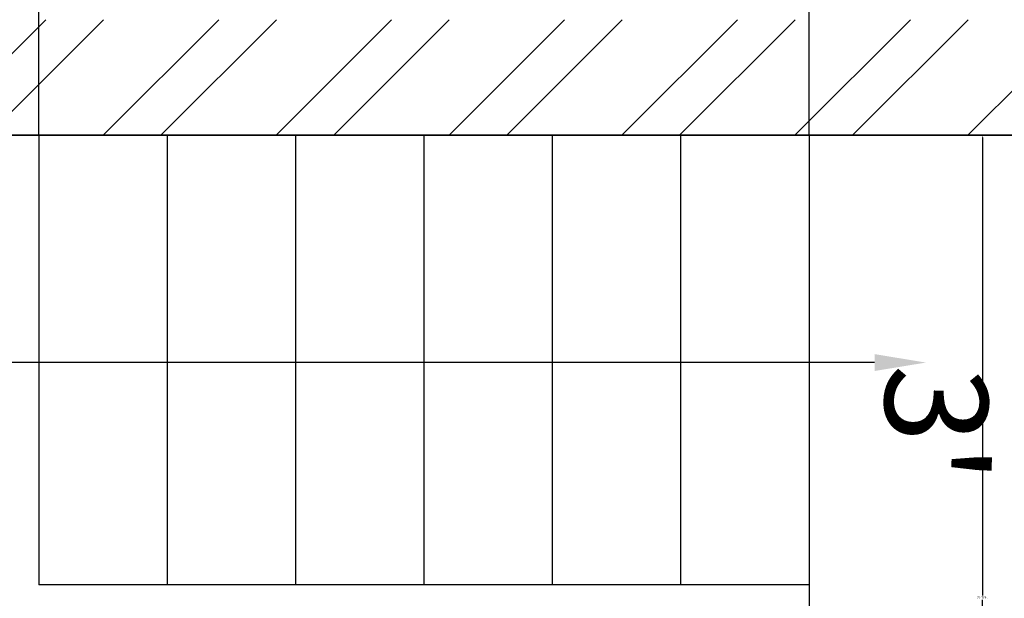
# Model space of a CAD drawing. Units: inches. Extents: x 2166 to 3588, y 1959 to 2628.
# Tile 10 of 13: x 3457 to 3534, y 2067 to 2112. Entities that reach past the tile are written whole.
import ezdxf
from ezdxf import colors
from ezdxf.entities.mleader import LeaderData, LeaderLine
from ezdxf.math import Vec2, Vec3

# ---------------------------------------------------------------- set-up
doc = ezdxf.new("R2010")
doc.units = ezdxf.units.IN
for name, color, linetype, lineweight in [('A-ANNO-DIMS', 2, 'Continuous', 18), ('A-ANNO-SYMB', 136, 'Continuous', 18), ('A-AREA-IDEN', 170, 'Continuous', 18), ('A-WALL-PATT', 20, 'Continuous', 13), ('Staircase', 136, 'Continuous', 25), ('WALL', 40, 'Continuous', 35)]:
    doc.layers.add(name, color=color, linetype=linetype, lineweight=lineweight)
doc.styles.get("Standard").update_dxf_attribs({"font": 'arial.ttf'})
doc.dimstyles.get("Standard").update_dxf_attribs({"dimtxt": 0.18, "dimasz": 0.18, "dimexe": 0.18, "dimexo": 0.0625, "dimgap": 0.09, "dimtad": 0, "dimtih": 1, "dimtoh": 1, "dimdec": 4, "dimzin": 0, "dimdsep": 46, "dimtxsty": 'Standard', "dimcen": 0.09, "dimadec": 0, "dimazin": 0, "dimtfac": 1, "dimtdec": 4, "dimtofl": 0, "dimtmove": 0, "dimatfit": 3, "dimfxl": 1, "dimtolj": 1, "dimtzin": 0, "dimarcsym": 0})

# ---------------------------------------------------------------- blocks, each defined once
blk = doc.blocks.new('STAIR-RETURN-FLIGHTS')
for p, q in [((30, 72), (30, 37)), ((40, 72), (40, 37)), ((50, 72), (50, 37)), ((60, 72), (60, 37)), ((70, 72), (70, 37)), ((80, 72), (80, 37)), ((90, 72), (90, 0)), ((90, 37), (30, 37))]:
    blk.add_line(p, q)
blk = doc.blocks.new('*D18')
at = {"layer": 'A-ANNO-DIMS', "color": 0, "lineweight": -2, "transparency": 16777216}
for p, q in [((3518.533, 2102.979), (3532.151, 2102.979)), ((3531.971, 2102.799), (3531.971, 2067.159)), ((3531.971, 2031.159), (3531.971, 2066.799)), ((3518.533, 2030.979), (3532.151, 2030.979))]:
    blk.add_line(p, q, dxfattribs=at)
at = {"layer": 'A-ANNO-DIMS', "color": 0, "transparency": 16777216}
for points in [[(3531.941, 2102.799), (3532.001, 2102.799), (3531.971, 2102.979)], [(3531.941, 2031.159), (3532.001, 2031.159), (3531.971, 2030.979)]]:
    blk.add_solid(points, dxfattribs=at)
at = {"layer": 'Defpoints', "color": 0, "transparency": 16777216}
for p in [(3518.471, 2102.979), (3531.971, 2102.979), (3518.471, 2030.979)]:
    blk.add_point(p, dxfattribs=at)
at = {"layer": 'A-ANNO-DIMS', "color": 0, "transparency": 16777216, "insert": (3531.971, 2066.979), "char_height": 0.18, "attachment_point": 5}
blk.add_mtext('\\A1;72 TYP.', dxfattribs=at)
blk = doc.blocks.new('*D52')
at = {"layer": 'A-ANNO-DIMS', "color": 0, "lineweight": -2, "transparency": 16777216}
for p, q in [((3458.471, 2103.041), (3458.471, 2127.909)), ((3458.651, 2127.729), (3488.251, 2127.729)), ((3518.291, 2127.729), (3488.69, 2127.729)), ((3518.471, 2103.041), (3518.471, 2127.909))]:
    blk.add_line(p, q, dxfattribs=at)
at = {"layer": 'A-ANNO-DIMS', "color": 0, "transparency": 16777216}
for points in [[(3458.651, 2127.759), (3458.651, 2127.699), (3458.471, 2127.729)], [(3518.291, 2127.759), (3518.291, 2127.699), (3518.471, 2127.729)]]:
    blk.add_solid(points, dxfattribs=at)
at = {"layer": 'Defpoints', "color": 0, "transparency": 16777216}
for p in [(3518.471, 2127.729), (3458.471, 2102.979), (3518.471, 2102.979)]:
    blk.add_point(p, dxfattribs=at)
at = {"layer": 'A-ANNO-DIMS', "color": 0, "transparency": 16777216, "insert": (3488.471, 2127.729), "char_height": 0.18, "attachment_point": 5}
blk.add_mtext('\\A1;60', dxfattribs=at)

msp = doc.modelspace()

# ---------------------------------------------------------------- hatches: boundary and pattern name
at = {"layer": 'A-WALL-PATT'}
h = msp.add_hatch(dxfattribs=at)
h.set_pattern_fill('ANSI32', color=256)
h.paths.add_polyline_path([(3563.471, 2429.979), (3227.471, 2429.979), (3227.471, 2021.979), (3563.471, 2021.979)])
h.paths.add_polyline_path([(3236.471, 2420.979), (3554.471, 2420.979), (3554.471, 2111.979), (3236.471, 2111.979)], flags=16)
h.paths.add_polyline_path([(3236.471, 2102.979), (3554.471, 2102.979), (3554.471, 2030.979), (3236.471, 2030.979)], flags=16)
h.paths.add_polyline_path([(3518.471, 2085.283), (3518.471, 2067.979), (3458.471, 2067.979), (3458.471, 2085.283)], flags=0)
h.paths.add_polyline_path([(3434.656, 2082.283), (3442.194, 2082.283), (3442.194, 2087.514), (3434.656, 2087.514)], flags=8)
h.paths.add_polyline_path([(3522.671, 2094.512), (3521.752, 2052.984), (3545.541, 2052.457), (3546.46, 2093.986)], flags=8)

# ---------------------------------------------------------------- linework, layer by layer
at = {"layer": 'WALL'}
msp.add_line((3554.471, 2102.979), (3236.471, 2102.979), dxfattribs=at)

# ---------------------------------------------------------------- block references
at = {"layer": 'Staircase'}
msp.add_blockref('STAIR-RETURN-FLIGHTS', (3428.471, 2030.979), dxfattribs=at)

# ---------------------------------------------------------------- texts
at = {"layer": 'A-AREA-IDEN', "insert": (3545.955, 2091.996), "char_height": 8, "attachment_point": 1, "rotation": 268.73191}
msp.add_mtext_dynamic_manual_height_columns("{\\Fsuperos|c0;LANDING\\P   3'}", width=58.85395, gutter_width=12.5, heights=[0], dxfattribs=at)

# ---------------------------------------------------------------- dimensions: what is measured, and where the dimension line sits
at = {"layer": 'A-ANNO-DIMS'}
dim = msp.add_linear_dim(base=(3518.471, 2127.729), p1=(3458.471, 2102.979), p2=(3518.471, 2102.979), dimstyle='Standard', override={"dimdec": 0, "dimlfac": 1, "dimrnd": 0, "dimzin": 0, "dimdsep": 46, "dimlunit": 2}, dxfattribs=at)
dim.commit()
dim.dimension.update_dxf_attribs({"geometry": '*D52', "text_midpoint": (3488.471, 2127.729)})
dim = msp.add_linear_dim(base=(3531.971, 2102.979), p1=(3518.471, 2030.979), p2=(3518.471, 2102.979), angle=90, text='<> TYP.', dimstyle='Standard', override={"dimdec": 0, "dimlfac": 1, "dimrnd": 0, "dimzin": 0, "dimdsep": 46, "dimlunit": 2}, dxfattribs=at)
dim.commit()
dim.dimension.update_dxf_attribs({"geometry": '*D18', "text_midpoint": (3531.971, 2066.979)})

# ---------------------------------------------------------------- leaders
at = {"layer": 'A-ANNO-SYMB'}
ml = msp.add_multileader_mtext('Standard', dxfattribs=at)
ml.set_content('{\\Fsuperos|c0;UP}', color=256)
ml.set_leader_properties()
ml.build(insert=Vec2(0, 0))
ctx = ml.context
ctx.base_point, ctx.plane_origin = Vec3(3433.656, 2085.283), Vec3(3527.576, 2085.283)
ctx.text_align_type = 2
notes = []
notes.append((ctx, [(0, (1, 1, 0), (3451.194, 2085.283), (-1, 0), 8, [(0, [(3527.576, 2085.283)], 0, [])])]))
ctx.mtext.insert, ctx.mtext.alignment, ctx.mtext.flow_direction = Vec3(3441.194, 2087.283), 3, 5
for ctx, leaders in notes:
    for number, flags, end, landing, length, lines in leaders:
        leader = LeaderData()
        leader.index, (leader.has_last_leader_line, leader.has_dogleg_vector, leader.attachment_direction) = number, flags
        leader.last_leader_point, leader.dogleg_vector, leader.dogleg_length = Vec3(end), Vec3(landing), length
        for number, points, colour, breaks in lines:
            line = LeaderLine()
            line.index, line.vertices, line.color, line.breaks = number, Vec3.list(points), colors.encode_raw_color(colour), breaks
            leader.lines.append(line)
        ctx.leaders.append(leader)

doc.saveas('drawing.dxf')
